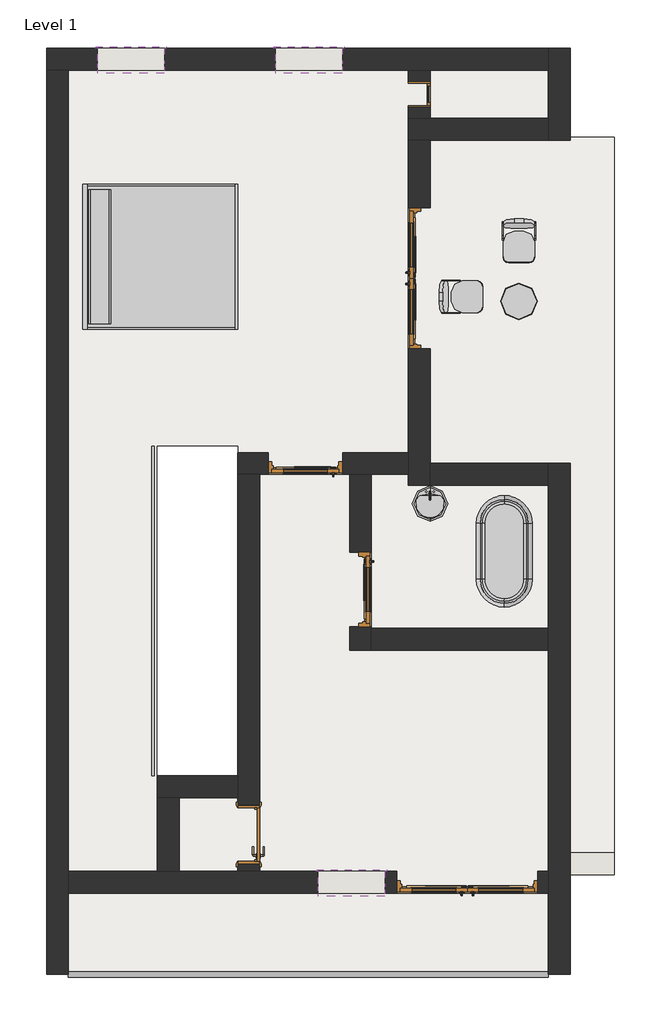
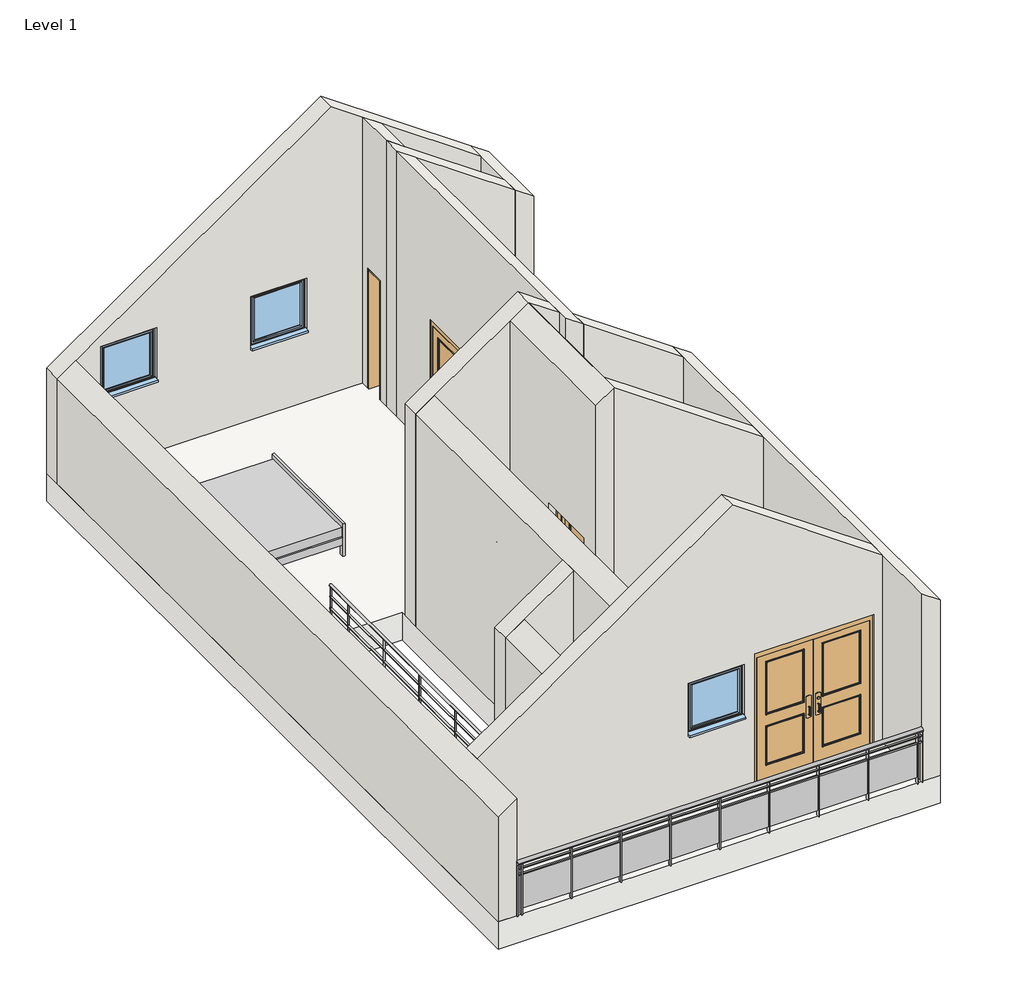
# One storey: 16 walls, 6 doors, 4 furniture elements, 3 windows, 2 flow terminals, 2 railings, 1 slab.
"""IFC4 building model written with IfcOpenShell, lengths in millimetres."""

from ifc_helpers import new_model, si_unit, point, frame, frame_2d, origin, place, context, project, spatial, polyline, circle_curve, ellipse_curve, trimmed, segment, composite_curve, outline, extrude, faceted_brep, transform, mapped, element, save
from ifc_brep_helpers import plane_surface, extruded_surface, advanced_brep
from components import door_9a5dd369, door_exterior_double_two_lite_door_exterior_double_two_lite_aa7d30b3, door_exterior_double_two_lite_door_exterior_double_two_lite_6b883914, door_exterior_double_two_lite_door_exterior_double_two_lite_037690dd, door_exterior_single_two_lite_door_exterior_single_two_lite_eb677f4d, doors_intsgl_810x2110mm_8206dd41, flow_terminal_a43f4bde, flow_terminal_0c5ffde2, furniture_b8e5f23d, furniture_eb3a3c23, furniture_9d41381f, windows_sgl_plain_910x910mm_cb8bb1e6

model = new_model("IFC4")

# Units and contexts
model_context = context("Model", 3, world=origin())
ifc_project = project(units=[si_unit("LENGTHUNIT", "METRE", prefix="MILLI")], contexts=[model_context])

# Site, building, storey
site = spatial("IfcSite", under=ifc_project)
building = spatial("IfcBuilding", under=site)
storey = spatial("IfcBuildingStorey", under=building, Name="Level 1", Elevation=3200.0)

# Doors
placement = place(None, origin())
door_shape = door_9a5dd369(model_context)
element("IfcDoor", 1, ObjectType="12\" x 80\"", at=placement, inside=storey, context=model_context, shape_type="MappedRepresentation", body=[
    mapped(door_shape, transform((-3132.0250057, 19503.7490528, 3200.0), x_axis=(0.0, -1.0, 0.0), y_axis=(1.0, 0.0, 0.0), z_axis=(0.0, 0.0, 1.0))),
])
door_exterior_double_two_lite_door_exterior_double_two_lite_shape = door_exterior_double_two_lite_door_exterior_double_two_lite_aa7d30b3(model_context)
door_exterior_double_two_lite_door_exterior_double_two_lite_2_shape = door_exterior_double_two_lite_door_exterior_double_two_lite_6b883914(model_context)
door_exterior_double_two_lite_door_exterior_double_two_lite_3_shape = door_exterior_double_two_lite_door_exterior_double_two_lite_037690dd(model_context)
element("IfcDoor", 2, ObjectType="Door-Exterior-Double-Two_Lite : Door-Exterior-Double-Two_Lite", at=placement, inside=storey, context=model_context, shape_type="MappedRepresentation", body=[
    mapped(door_exterior_double_two_lite_door_exterior_double_two_lite_shape, transform((-3128.8500057, 16990.7490528, 3200.0), x_axis=(0.0, 1.0, 0.0), y_axis=(-1.0, 0.0, 0.0), z_axis=(0.0, 0.0, 1.0))),
    mapped(door_exterior_double_two_lite_door_exterior_double_two_lite_2_shape, transform((-3128.8500057, 16990.7490528, 3200.0), x_axis=(0.0, 1.0, 0.0), y_axis=(-1.0, 0.0, 0.0), z_axis=(0.0, 0.0, 1.0))),
    mapped(door_exterior_double_two_lite_door_exterior_double_two_lite_3_shape, transform((-3128.8500057, 16990.7490528, 3200.0), x_axis=(0.0, 1.0, 0.0), y_axis=(-1.0, 0.0, 0.0), z_axis=(0.0, 0.0, 1.0))),
])
element("IfcDoor", 3, ObjectType="Door-Exterior-Double-Two_Lite : Door-Exterior-Double-Two_Lite", at=placement, inside=storey, context=model_context, shape_type="MappedRepresentation", body=[
    mapped(door_exterior_double_two_lite_door_exterior_double_two_lite_shape, transform((-2475.6750057, 8741.3490528, 3200.0), x_axis=(-1.0, 0.0, 0.0), y_axis=(0.0, -1.0, 0.0), z_axis=(0.0, 0.0, 1.0))),
    mapped(door_exterior_double_two_lite_door_exterior_double_two_lite_2_shape, transform((-2475.6750057, 8741.3490528, 3200.0), x_axis=(-1.0, 0.0, 0.0), y_axis=(0.0, -1.0, 0.0), z_axis=(0.0, 0.0, 1.0))),
    mapped(door_exterior_double_two_lite_door_exterior_double_two_lite_3_shape, transform((-2475.6750057, 8741.3490528, 3200.0), x_axis=(-1.0, 0.0, 0.0), y_axis=(0.0, -1.0, 0.0), z_axis=(0.0, 0.0, 1.0))),
])
door_exterior_single_two_lite_door_exterior_single_two_lite_shape = door_exterior_single_two_lite_door_exterior_single_two_lite_eb677f4d(model_context)
element("IfcDoor", 4, ObjectType="Door-Exterior-Single-Two_Lite : Door-Exterior-Single-Two_Lite", at=placement, inside=storey, context=model_context, shape_type="MappedRepresentation", body=[
    mapped(door_exterior_single_two_lite_door_exterior_single_two_lite_shape, transform((-4688.1750057, 14466.3490528, 3200.0), x_axis=(-1.0, 0.0, 0.0), y_axis=(0.0, -1.0, 0.0), z_axis=(0.0, 0.0, 1.0))),
])
element("IfcDoor", 5, ObjectType="Door-Exterior-Single-Two_Lite : Door-Exterior-Single-Two_Lite", at=placement, inside=storey, context=model_context, shape_type="MappedRepresentation", body=[
    mapped(door_exterior_single_two_lite_door_exterior_single_two_lite_shape, transform((-3941.5500057, 12737.0490528, 3200.0), x_axis=(0.0, -1.0, 0.0), y_axis=(1.0, 0.0, 0.0), z_axis=(0.0, 0.0, 1.0))),
])
doors_intsgl_810x2110mm_shape = doors_intsgl_810x2110mm_8206dd41(model_context)
element("IfcDoor", 6, ObjectType="Doors_IntSgl : 810x2110mm", at=placement, inside=storey, context=model_context, shape_type="MappedRepresentation", body=[
    mapped(doors_intsgl_810x2110mm_shape, transform((-5460.2000057, 9388.7490528, 3200.0), x_axis=(0.0, 1.0, 0.0), y_axis=(-1.0, 0.0, 0.0), z_axis=(0.0, 0.0, 1.0))),
])

# Flow terminals
flow_terminal_shape = flow_terminal_a43f4bde(model_context)
element("IfcFlowTerminal", 7, ObjectType="Sink Vanity-Round : 19\" x 19\"", at=placement, inside=storey, context=model_context, shape_type="MappedRepresentation", body=[
    mapped(flow_terminal_shape, transform((-3081.8517463, 13827.6587105, 3200.0), x_axis=(1.0, 0.0, 0.0), y_axis=(0.0, 1.0, 0.0), z_axis=(0.0, 0.0, 1.0))),
])
flow_terminal_2_shape = flow_terminal_0c5ffde2(model_context)
element("IfcFlowTerminal", 8, ObjectType="Tub-Free Standing-3D : 30\" x 60\"", at=placement, inside=storey, context=model_context, shape_type="MappedRepresentation", body=[
    mapped(flow_terminal_2_shape, transform((-1970.2000057, 13259.9990528, 3200.0), x_axis=(1.0, 0.0, 0.0), y_axis=(0.0, 1.0, 0.0), z_axis=(0.0, 0.0, 1.0))),
])

# Furniture
furniture_shape = furniture_b8e5f23d(model_context)
element("IfcFurniture", 9, ObjectType="Bed-Shaker : King 78\" x 83\"", at=placement, inside=storey, context=model_context, shape_type="MappedRepresentation", body=[
    mapped(furniture_shape, transform((-7718.4000057, 17303.4490528, 3200.0), x_axis=(0.0, 1.0, 0.0), y_axis=(-1.0, 0.0, 0.0), z_axis=(0.0, 0.0, 1.0))),
])
furniture_2_shape = furniture_eb3a3c23(model_context)
element("IfcFurniture", 10, ObjectType="Seating-Auditorium : 18\" x 24\" x 30\"", at=placement, inside=storey, context=model_context, shape_type="MappedRepresentation", body=[
    mapped(furniture_2_shape, transform((-2760.0754155, 16899.3269216, 3200.0), x_axis=(0.0, -1.0, 0.0), y_axis=(1.0, 0.0, 0.0), z_axis=(0.0, 0.0, 1.0))),
])
element("IfcFurniture", 11, ObjectType="Seating-Auditorium : 18\" x 24\" x 30\"", at=placement, inside=storey, context=model_context, shape_type="MappedRepresentation", body=[
    mapped(furniture_2_shape, transform((-1609.4721368, 17699.8744626, 3200.0), x_axis=(-1.0, 0.0, 0.0), y_axis=(0.0, -1.0, 0.0), z_axis=(0.0, 0.0, 1.0))),
])
furniture_3_shape = furniture_9d41381f(model_context)
element("IfcFurniture", 12, ObjectType="Table-Trio End : 20\" Diameter", at=placement, inside=storey, context=model_context, shape_type="MappedRepresentation", body=[
    mapped(furniture_3_shape, transform((-1770.2000057, 16674.9990528, 3200.0), x_axis=(1.0, 0.0, 0.0), y_axis=(0.0, 1.0, 0.0), z_axis=(0.0, 0.0, 1.0))),
])

# Railings
element("IfcRailing", 13, ObjectType="900mm_Pipe", at=placement, inside=storey, context=model_context, shape_type="SweptSolid", body=[
    extrude(outline(composite_curve([segment(trimmed(circle_curve(frame_2d((4080.0, -6770.2000057)), 20.0), [point((4080.0, -6750.2000057))], [point((4080.0, -6790.2000057))], False, "CARTESIAN"), True, "CONTINUOUS"), segment(trimmed(circle_curve(frame_2d((4080.0, -6770.2000057)), 20.0), [point((4080.0, -6790.2000057))], [point((4080.0, -6750.2000057))], False, "CARTESIAN"), True, "CONTINUOUS")], self_intersect=False)), frame((0.0, 10192.4990528, 0.0), z_axis=(0.0, 1.0, 0.0), x_axis=(0.0, 0.0, 1.0)), (0.0, 0.0, 1.0), 4500.0),
    extrude(outline(composite_curve([segment(trimmed(circle_curve(frame_2d((3885.0, -6770.2000057)), 15.0), [point((3885.0, -6785.2000057))], [point((3885.0, -6755.2000057))], False, "CARTESIAN"), True, "CONTINUOUS"), segment(trimmed(circle_curve(frame_2d((3885.0, -6770.2000057)), 15.0), [point((3885.0, -6755.2000057))], [point((3885.0, -6785.2000057))], False, "CARTESIAN"), True, "CONTINUOUS")], self_intersect=False)), frame((0.0, 10192.4990528, 0.0), z_axis=(0.0, 1.0, 0.0), x_axis=(0.0, 0.0, 1.0)), (0.0, 0.0, 1.0), 4500.0),
    extrude(outline(composite_curve([segment(trimmed(circle_curve(frame_2d((3685.0, -6770.2000057)), 15.0), [point((3685.0, -6785.2000057))], [point((3685.0, -6755.2000057))], False, "CARTESIAN"), True, "CONTINUOUS"), segment(trimmed(circle_curve(frame_2d((3685.0, -6770.2000057)), 15.0), [point((3685.0, -6755.2000057))], [point((3685.0, -6785.2000057))], False, "CARTESIAN"), True, "CONTINUOUS")], self_intersect=False)), frame((0.0, 10192.4990528, 0.0), z_axis=(0.0, 1.0, 0.0), x_axis=(0.0, 0.0, 1.0)), (0.0, 0.0, 1.0), 4500.0),
    extrude(outline(composite_curve([segment(trimmed(circle_curve(frame_2d((3485.0, -6770.2000057)), 15.0), [point((3485.0, -6785.2000057))], [point((3485.0, -6755.2000057))], False, "CARTESIAN"), True, "CONTINUOUS"), segment(trimmed(circle_curve(frame_2d((3485.0, -6770.2000057)), 15.0), [point((3485.0, -6755.2000057))], [point((3485.0, -6785.2000057))], False, "CARTESIAN"), True, "CONTINUOUS")], self_intersect=False)), frame((0.0, 10192.4990528, 0.0), z_axis=(0.0, 1.0, 0.0), x_axis=(0.0, 0.0, 1.0)), (0.0, 0.0, 1.0), 4500.0),
    extrude(outline(composite_curve([segment(trimmed(circle_curve(frame_2d((3285.0, -6770.2000057)), 15.0), [point((3285.0, -6785.2000057))], [point((3285.0, -6755.2000057))], False, "CARTESIAN"), True, "CONTINUOUS"), segment(trimmed(circle_curve(frame_2d((3285.0, -6770.2000057)), 15.0), [point((3285.0, -6755.2000057))], [point((3285.0, -6785.2000057))], False, "CARTESIAN"), True, "CONTINUOUS")], self_intersect=False)), frame((0.0, 10192.4990528, 0.0), z_axis=(0.0, 1.0, 0.0), x_axis=(0.0, 0.0, 1.0)), (0.0, 0.0, 1.0), 4500.0),
    extrude(outline(composite_curve([segment(trimmed(circle_curve(frame_2d((-6770.2000057, 14192.4990528)), 12.5), [point((-6782.7000057, 14192.4990528))], [point((-6757.7000057, 14192.4990528))], False, "CARTESIAN"), True, "CONTINUOUS"), segment(trimmed(circle_curve(frame_2d((-6770.2000057, 14192.4990528)), 12.5), [point((-6757.7000057, 14192.4990528))], [point((-6782.7000057, 14192.4990528))], False, "CARTESIAN"), True, "CONTINUOUS")], self_intersect=False)), frame((0.0, 0.0, 3200.0), z_axis=(0.0, 0.0, 1.0), x_axis=(1.0, 0.0, 0.0)), (0.0, 0.0, 1.0), 860.0),
    extrude(outline(composite_curve([segment(trimmed(circle_curve(frame_2d((-6770.2000057, 13192.4990528)), 12.5), [point((-6782.7000057, 13192.4990528))], [point((-6757.7000057, 13192.4990528))], False, "CARTESIAN"), True, "CONTINUOUS"), segment(trimmed(circle_curve(frame_2d((-6770.2000057, 13192.4990528)), 12.5), [point((-6757.7000057, 13192.4990528))], [point((-6782.7000057, 13192.4990528))], False, "CARTESIAN"), True, "CONTINUOUS")], self_intersect=False)), frame((0.0, 0.0, 3200.0), z_axis=(0.0, 0.0, 1.0), x_axis=(1.0, 0.0, 0.0)), (0.0, 0.0, 1.0), 860.0),
    extrude(outline(composite_curve([segment(trimmed(circle_curve(frame_2d((-6770.2000057, 12192.4990528)), 12.5), [point((-6782.7000057, 12192.4990528))], [point((-6757.7000057, 12192.4990528))], False, "CARTESIAN"), True, "CONTINUOUS"), segment(trimmed(circle_curve(frame_2d((-6770.2000057, 12192.4990528)), 12.5), [point((-6757.7000057, 12192.4990528))], [point((-6782.7000057, 12192.4990528))], False, "CARTESIAN"), True, "CONTINUOUS")], self_intersect=False)), frame((0.0, 0.0, 3200.0), z_axis=(0.0, 0.0, 1.0), x_axis=(1.0, 0.0, 0.0)), (0.0, 0.0, 1.0), 860.0),
    extrude(outline(composite_curve([segment(trimmed(circle_curve(frame_2d((-6770.2000057, 11192.4990528)), 12.5), [point((-6782.7000057, 11192.4990528))], [point((-6757.7000057, 11192.4990528))], False, "CARTESIAN"), True, "CONTINUOUS"), segment(trimmed(circle_curve(frame_2d((-6770.2000057, 11192.4990528)), 12.5), [point((-6757.7000057, 11192.4990528))], [point((-6782.7000057, 11192.4990528))], False, "CARTESIAN"), True, "CONTINUOUS")], self_intersect=False)), frame((0.0, 0.0, 3200.0), z_axis=(0.0, 0.0, 1.0), x_axis=(1.0, 0.0, 0.0)), (0.0, 0.0, 1.0), 860.0),
    extrude(outline(composite_curve([segment(trimmed(circle_curve(frame_2d((-6770.2000057, 14679.9990528)), 12.5), [point((-6782.7000057, 14679.9990528))], [point((-6757.7000057, 14679.9990528))], False, "CARTESIAN"), True, "CONTINUOUS"), segment(trimmed(circle_curve(frame_2d((-6770.2000057, 14679.9990528)), 12.5), [point((-6757.7000057, 14679.9990528))], [point((-6782.7000057, 14679.9990528))], False, "CARTESIAN"), True, "CONTINUOUS")], self_intersect=False)), frame((0.0, 0.0, 3200.0), z_axis=(0.0, 0.0, 1.0), x_axis=(1.0, 0.0, 0.0)), (0.0, 0.0, 1.0), 860.0),
    extrude(outline(composite_curve([segment(trimmed(circle_curve(frame_2d((-6770.2000057, 10204.9990528)), 12.5), [point((-6782.7000057, 10204.9990528))], [point((-6757.7000057, 10204.9990528))], False, "CARTESIAN"), True, "CONTINUOUS"), segment(trimmed(circle_curve(frame_2d((-6770.2000057, 10204.9990528)), 12.5), [point((-6757.7000057, 10204.9990528))], [point((-6782.7000057, 10204.9990528))], False, "CARTESIAN"), True, "CONTINUOUS")], self_intersect=False)), frame((0.0, 0.0, 3200.0), z_axis=(0.0, 0.0, 1.0), x_axis=(1.0, 0.0, 0.0)), (0.0, 0.0, 1.0), 860.0),
])
element("IfcRailing", 14, ObjectType="Glass_Panel-Bottom_Fill", at=placement, inside=storey, context=model_context, shape_type="SolidModel", body=[
    advanced_brep(
    [(-7925.2000057, 7516.889818, 4100.0), (-7925.2000057, 7436.889818, 4100.0), (-1370.2000057, 7516.889818, 4100.0), (-1370.2000057, 7436.889818, 4100.0)],
    [
        (0, 1, ellipse_curve(frame((-7925.2000057, 7476.889818, 4100.0), z_axis=(-1.0, 0.0, 0.0), x_axis=(0.0, -1.0, 0.0)), 40.0, 30.0)),
        (1, 0, ellipse_curve(frame((-7925.2000057, 7476.889818, 4100.0), z_axis=(-1.0, 0.0, 0.0), x_axis=(0.0, -1.0, 0.0)), 40.0, 30.0)),
        (2, 3, ellipse_curve(frame((-1370.2000057, 7476.889818, 4100.0), z_axis=(1.0, 0.0, 0.0), x_axis=(0.0, -1.0, 0.0)), 40.0, 30.0)),
        (3, 2, ellipse_curve(frame((-1370.2000057, 7476.889818, 4100.0), z_axis=(1.0, 0.0, 0.0), x_axis=(0.0, -1.0, 0.0)), 40.0, 30.0)),
        (0, 2),
        (3, 1),
    ],
    [
        plane_surface(frame((-7925.2000057, 7476.889818, 4100.0), z_axis=(-1.0, 0.0, 0.0), x_axis=(0.0, 1.0, 0.0))),
        plane_surface(frame((-1370.2000057, 7476.889818, 4100.0), z_axis=(1.0, 0.0, 0.0), x_axis=(0.0, 1.0, 0.0))),
        extruded_surface(trimmed(ellipse_curve(frame((-1370.2000057, 7476.889818, 4100.0), z_axis=(-1.0, 0.0, 0.0), x_axis=(0.0, -1.0, 0.0)), 40.0, 30.0), [point((-1370.2000057, 7516.889818, 4100.0))], [point((-1370.2000057, 7436.889818, 4100.0))], True, "CARTESIAN"), (-6555.0, 0.0, 0.0), 6555.0),
        extruded_surface(trimmed(ellipse_curve(frame((-1370.2000057, 7476.889818, 4100.0), z_axis=(-1.0, 0.0, 0.0), x_axis=(0.0, -1.0, 0.0)), 40.0, 30.0), [point((-1370.2000057, 7436.889818, 4100.0))], [point((-1370.2000057, 7516.889818, 4100.0))], True, "CARTESIAN"), (-6555.0, 0.0, 0.0), 6555.0),
    ],
    [
        (0, [[1, 2]]),
        (1, [[3, 4]]),
        (2, [[-1, 5, -4, 6]]),
        (3, [[-2, -6, -3, -5]]),
    ],
),
    extrude(outline(polyline([(-7925.2000057, 7467.4990528), (-7925.2000057, 7487.4990528), (-1370.2000057, 7487.4990528), (-1370.2000057, 7467.4990528), (-7925.2000057, 7467.4990528)])), frame((0.0, 0.0, 3980.0), z_axis=(0.0, 0.0, 1.0), x_axis=(1.0, 0.0, 0.0)), (0.0, 0.0, 1.0), 20.0),
    extrude(outline(polyline([(-7925.2000057, 7467.4990528), (-7925.2000057, 7487.4990528), (-1370.2000057, 7487.4990528), (-1370.2000057, 7467.4990528), (-7925.2000057, 7467.4990528)])), frame((0.0, 0.0, 3880.0), z_axis=(0.0, 0.0, 1.0), x_axis=(1.0, 0.0, 0.0)), (0.0, 0.0, 1.0), 20.0),
    extrude(outline(polyline([(-1453.7000057, 7502.4990528), (-1441.7000057, 7502.4990528), (-1441.7000057, 7452.4990528), (-1453.7000057, 7452.4990528), (-1453.7000057, 7502.4990528)])), frame((0.0, 0.0, 3200.0), z_axis=(0.0, 0.0, 1.0), x_axis=(1.0, 0.0, 0.0)), (0.0, 0.0, 1.0), 870.0),
    extrude(outline(polyline([(-2247.7000057, 7475.7742427), (-1447.7000057, 7475.7742427), (-1447.7000057, 7470.7742427), (-2247.7000057, 7470.7742427), (-2247.7000057, 7475.7742427)])), frame((0.0, 0.0, 3300.0), z_axis=(0.0, 0.0, 1.0), x_axis=(1.0, 0.0, 0.0)), (0.0, 0.0, 1.0), 580.0),
    extrude(outline(polyline([(-2253.7000057, 7502.4990528), (-2241.7000057, 7502.4990528), (-2241.7000057, 7452.4990528), (-2253.7000057, 7452.4990528), (-2253.7000057, 7502.4990528)])), frame((0.0, 0.0, 3200.0), z_axis=(0.0, 0.0, 1.0), x_axis=(1.0, 0.0, 0.0)), (0.0, 0.0, 1.0), 870.0),
    extrude(outline(polyline([(-3047.7000057, 7475.7742427), (-2247.7000057, 7475.7742427), (-2247.7000057, 7470.7742427), (-3047.7000057, 7470.7742427), (-3047.7000057, 7475.7742427)])), frame((0.0, 0.0, 3300.0), z_axis=(0.0, 0.0, 1.0), x_axis=(1.0, 0.0, 0.0)), (0.0, 0.0, 1.0), 580.0),
    extrude(outline(polyline([(-3053.7000057, 7502.4990528), (-3041.7000057, 7502.4990528), (-3041.7000057, 7452.4990528), (-3053.7000057, 7452.4990528), (-3053.7000057, 7502.4990528)])), frame((0.0, 0.0, 3200.0), z_axis=(0.0, 0.0, 1.0), x_axis=(1.0, 0.0, 0.0)), (0.0, 0.0, 1.0), 870.0),
    extrude(outline(polyline([(-3847.7000057, 7475.7742427), (-3047.7000057, 7475.7742427), (-3047.7000057, 7470.7742427), (-3847.7000057, 7470.7742427), (-3847.7000057, 7475.7742427)])), frame((0.0, 0.0, 3300.0), z_axis=(0.0, 0.0, 1.0), x_axis=(1.0, 0.0, 0.0)), (0.0, 0.0, 1.0), 580.0),
    extrude(outline(polyline([(-3853.7000057, 7502.4990528), (-3841.7000057, 7502.4990528), (-3841.7000057, 7452.4990528), (-3853.7000057, 7452.4990528), (-3853.7000057, 7502.4990528)])), frame((0.0, 0.0, 3200.0), z_axis=(0.0, 0.0, 1.0), x_axis=(1.0, 0.0, 0.0)), (0.0, 0.0, 1.0), 870.0),
    extrude(outline(polyline([(-4647.7000057, 7475.7742427), (-3847.7000057, 7475.7742427), (-3847.7000057, 7470.7742427), (-4647.7000057, 7470.7742427), (-4647.7000057, 7475.7742427)])), frame((0.0, 0.0, 3300.0), z_axis=(0.0, 0.0, 1.0), x_axis=(1.0, 0.0, 0.0)), (0.0, 0.0, 1.0), 580.0),
    extrude(outline(polyline([(-4653.7000057, 7502.4990528), (-4641.7000057, 7502.4990528), (-4641.7000057, 7452.4990528), (-4653.7000057, 7452.4990528), (-4653.7000057, 7502.4990528)])), frame((0.0, 0.0, 3200.0), z_axis=(0.0, 0.0, 1.0), x_axis=(1.0, 0.0, 0.0)), (0.0, 0.0, 1.0), 870.0),
    extrude(outline(polyline([(-5447.7000057, 7475.7742427), (-4647.7000057, 7475.7742427), (-4647.7000057, 7470.7742427), (-5447.7000057, 7470.7742427), (-5447.7000057, 7475.7742427)])), frame((0.0, 0.0, 3300.0), z_axis=(0.0, 0.0, 1.0), x_axis=(1.0, 0.0, 0.0)), (0.0, 0.0, 1.0), 580.0),
    extrude(outline(polyline([(-5453.7000057, 7502.4990528), (-5441.7000057, 7502.4990528), (-5441.7000057, 7452.4990528), (-5453.7000057, 7452.4990528), (-5453.7000057, 7502.4990528)])), frame((0.0, 0.0, 3200.0), z_axis=(0.0, 0.0, 1.0), x_axis=(1.0, 0.0, 0.0)), (0.0, 0.0, 1.0), 870.0),
    extrude(outline(polyline([(-6247.7000057, 7475.7742427), (-5447.7000057, 7475.7742427), (-5447.7000057, 7470.7742427), (-6247.7000057, 7470.7742427), (-6247.7000057, 7475.7742427)])), frame((0.0, 0.0, 3300.0), z_axis=(0.0, 0.0, 1.0), x_axis=(1.0, 0.0, 0.0)), (0.0, 0.0, 1.0), 580.0),
    extrude(outline(polyline([(-6253.7000057, 7502.4990528), (-6241.7000057, 7502.4990528), (-6241.7000057, 7452.4990528), (-6253.7000057, 7452.4990528), (-6253.7000057, 7502.4990528)])), frame((0.0, 0.0, 3200.0), z_axis=(0.0, 0.0, 1.0), x_axis=(1.0, 0.0, 0.0)), (0.0, 0.0, 1.0), 870.0),
    extrude(outline(polyline([(-7047.7000057, 7475.7742427), (-6247.7000057, 7475.7742427), (-6247.7000057, 7470.7742427), (-7047.7000057, 7470.7742427), (-7047.7000057, 7475.7742427)])), frame((0.0, 0.0, 3300.0), z_axis=(0.0, 0.0, 1.0), x_axis=(1.0, 0.0, 0.0)), (0.0, 0.0, 1.0), 580.0),
    extrude(outline(polyline([(-7053.7000057, 7502.4990528), (-7041.7000057, 7502.4990528), (-7041.7000057, 7452.4990528), (-7053.7000057, 7452.4990528), (-7053.7000057, 7502.4990528)])), frame((0.0, 0.0, 3200.0), z_axis=(0.0, 0.0, 1.0), x_axis=(1.0, 0.0, 0.0)), (0.0, 0.0, 1.0), 870.0),
    extrude(outline(polyline([(-7847.7000057, 7475.7742427), (-7047.7000057, 7475.7742427), (-7047.7000057, 7470.7742427), (-7847.7000057, 7470.7742427), (-7847.7000057, 7475.7742427)])), frame((0.0, 0.0, 3300.0), z_axis=(0.0, 0.0, 1.0), x_axis=(1.0, 0.0, 0.0)), (0.0, 0.0, 1.0), 580.0),
    extrude(outline(polyline([(-7853.7000057, 7502.4990528), (-7841.7000057, 7502.4990528), (-7841.7000057, 7452.4990528), (-7853.7000057, 7452.4990528), (-7853.7000057, 7502.4990528)])), frame((0.0, 0.0, 3200.0), z_axis=(0.0, 0.0, 1.0), x_axis=(1.0, 0.0, 0.0)), (0.0, 0.0, 1.0), 870.0),
    extrude(outline(polyline([(-1378.2000057, 7502.4990528), (-1366.2000057, 7502.4990528), (-1366.2000057, 7452.4990528), (-1378.2000057, 7452.4990528), (-1378.2000057, 7502.4990528)])), frame((0.0, 0.0, 3200.0), z_axis=(0.0, 0.0, 1.0), x_axis=(1.0, 0.0, 0.0)), (0.0, 0.0, 1.0), 870.0),
    extrude(outline(polyline([(-7929.2000057, 7502.4990528), (-7917.2000057, 7502.4990528), (-7917.2000057, 7452.4990528), (-7929.2000057, 7452.4990528), (-7929.2000057, 7502.4990528)])), frame((0.0, 0.0, 3200.0), z_axis=(0.0, 0.0, 1.0), x_axis=(1.0, 0.0, 0.0)), (0.0, 0.0, 1.0), 870.0),
])

# Slab
element("IfcSlab", 15, ObjectType="floor generic 150mm", at=placement, inside=storey, context=model_context, shape_type="SweptSolid", body=[
    extrude(outline(polyline([(-8225.2000057, 20132.4990528), (-1070.2000057, 20132.4990528), (-1070.2000057, 18917.4990528), (-470.2000057, 18917.4990528), (-470.2000057, 8842.4990528), (-481.4492748, 8842.4990528), (-1070.2000057, 8842.4990528), (-1070.2000057, 7477.4990528), (-8225.2000057, 7477.4990528), (-8225.2000057, 20132.4990528)]), holes=[polyline([(-5610.2000057, 14692.4990528), (-6710.2000057, 14692.4990528), (-6710.2000057, 10192.4990528), (-5610.2000057, 10192.4990528), (-5610.2000057, 14692.4990528)])]), frame((0.0, 0.0, 2730.0), z_axis=(0.0, 0.0, 1.0), x_axis=(1.0, 0.0, 0.0)), (0.0, 0.0, 1.0), 470.0),
])

# Walls
element("IfcWall", 16, at=placement, inside=storey, context=model_context, shape_type="Brep", body=[
    faceted_brep([(-2985.2000057, 19832.4990528, 3200.0), (-2985.2000057, 19832.4990528, 7540.8974357), (-2985.2000057, 19174.9990528, 7540.8974357), (-2985.2000057, 19174.9990528, 3200.0), (-2985.2000057, 19325.9490528, 3200.0), (-2985.2000057, 19325.9490528, 5257.4), (-2985.2000057, 19681.5490528, 5257.4), (-2985.2000057, 19681.5490528, 3200.0), (-3285.2000057, 19832.4990528, 7750.9596971), (-3285.2000057, 19832.4990528, 3200.0), (-3285.2000057, 19681.5490528, 3200.0), (-3285.2000057, 19681.5490528, 5257.4), (-3285.2000057, 19325.9490528, 5257.4), (-3285.2000057, 19325.9490528, 3200.0), (-3285.2000057, 19174.9990528, 3200.0), (-3285.2000057, 19174.9990528, 7750.9596971)], [[[0, 1, 2, 3, 4, 5, 6, 7]], [[8, 9, 10, 11, 12, 13, 14, 15]], [[3, 14, 13, 4]], [[9, 0, 7, 10]], [[1, 0, 9, 8]], [[3, 2, 15, 14]], [[12, 5, 4, 13]], [[6, 11, 10, 7]], [[2, 1, 8, 15]], [[11, 6, 5, 12]]]),
])
element("IfcWall", 17, at=placement, inside=storey, context=model_context, shape_type="Brep", body=[
    faceted_brep([(-3285.2000057, 14609.9990528, 7750.9596971), (-3285.2000057, 14609.9990528, 3200.0), (-4180.1750057, 14609.9990528, 3200.0), (-4180.1750057, 14609.9990528, 5435.2), (-5196.1750057, 14609.9990528, 5435.2), (-5196.1750057, 14609.9990528, 3200.0), (-5610.2000057, 14609.9990528, 3200.0), (-5610.2000057, 14609.9990528, 6831.0427124), (-3790.8112016, 14609.9990528, 8104.9924679), (-3285.2000057, 14309.9990528, 3200.0), (-3285.2000057, 14309.9990528, 7750.9596971), (-3785.2000057, 14309.9990528, 8101.0634662), (-3790.8112016, 14309.9990528, 8104.9924679), (-4085.2000057, 14309.9990528, 7898.8592082), (-5310.2000057, 14309.9990528, 7041.1049739), (-5610.2000057, 14309.9990528, 6831.0427124), (-5610.2000057, 14309.9990528, 3200.0), (-5310.2000057, 14309.9990528, 3200.0), (-5196.1750057, 14309.9990528, 3200.0), (-5196.1750057, 14309.9990528, 5435.2), (-4180.1750057, 14309.9990528, 5435.2), (-4180.1750057, 14309.9990528, 3200.0), (-4085.2000057, 14309.9990528, 3200.0), (-3785.2000057, 14309.9990528, 3200.0)], [[[0, 1, 2, 3, 4, 5, 6, 7, 8]], [[9, 10, 11, 12, 13, 14, 15, 16, 17, 18, 19, 20, 21, 22, 23]], [[1, 9, 23, 22, 21, 2]], [[16, 6, 5, 18, 17]], [[1, 0, 10, 9]], [[7, 6, 16, 15]], [[4, 19, 18, 5]], [[20, 3, 2, 21]], [[10, 0, 8, 12, 11]], [[7, 15, 14, 13, 12, 8]], [[3, 20, 19, 4]]]),
])
element("IfcWall", 18, at=placement, inside=storey, context=model_context, shape_type="Brep", body=[
    faceted_brep([(-5610.2000057, 14309.9990528, 6831.0427124), (-5610.2000057, 14309.9990528, 3200.0), (-5610.2000057, 10192.4990528, 3200.0), (-5610.2000057, 9892.4990528, 3200.0), (-5610.2000057, 9793.7490528, 3200.0), (-5610.2000057, 9793.7490528, 5310.0), (-5610.2000057, 8983.7490528, 5310.0), (-5610.2000057, 8983.7490528, 3200.0), (-5610.2000057, 8884.9990528, 3200.0), (-5610.2000057, 8884.9990528, 6831.0427124), (-5610.2000057, 9892.4990528, 6831.0427124), (-5610.2000057, 10192.4990528, 6831.0427124), (-5310.2000057, 14309.9990528, 3200.0), (-5310.2000057, 14309.9990528, 7041.1049739), (-5310.2000057, 8884.9990528, 7041.1049739), (-5310.2000057, 8884.9990528, 3200.0), (-5310.2000057, 8983.7490528, 3200.0), (-5310.2000057, 8983.7490528, 5310.0), (-5310.2000057, 9793.7490528, 5310.0), (-5310.2000057, 9793.7490528, 3200.0)], [[[0, 1, 2, 3, 4, 5, 6, 7, 8, 9, 10, 11]], [[12, 13, 14, 15, 16, 17, 18, 19]], [[1, 12, 19, 4, 3, 2]], [[15, 8, 7, 16]], [[1, 0, 13, 12]], [[9, 8, 15, 14]], [[18, 5, 4, 19]], [[6, 17, 16, 7]], [[0, 11, 10, 9, 14, 13]], [[17, 6, 5, 18]]]),
])
element("IfcWall", 19, at=placement, inside=storey, context=model_context, shape_type="Brep", body=[
    faceted_brep([(-5610.2000057, 10192.4990528, 3200.0), (-6710.2000057, 10192.4990528, 3200.0), (-6710.2000057, 10192.4990528, 6060.8144204), (-5610.2000057, 10192.4990528, 6831.0427124), (-5610.2000057, 9892.4990528, 3200.0), (-5610.2000057, 9892.4990528, 6831.0427124), (-6410.2000057, 9892.4990528, 6270.8766819), (-6710.2000057, 9892.4990528, 6060.8144204), (-6710.2000057, 9892.4990528, 3200.0), (-6410.2000057, 9892.4990528, 3200.0)], [[[0, 1, 2, 3]], [[4, 5, 6, 7, 8, 9]], [[1, 0, 4, 9, 8]], [[0, 3, 5, 4]], [[2, 1, 8, 7]], [[3, 2, 7, 6, 5]]]),
])
element("IfcWall", 20, at=placement, inside=storey, context=model_context, shape_type="SweptSolid", body=[
    extrude(outline(polyline([(6060.8144204, -6710.2000057), (3200.0, -6710.2000057), (3200.0, -6410.2000057), (6270.8766819, -6410.2000057), (6060.8144204, -6710.2000057)])), frame((0.0, 8884.9990528, 0.0), z_axis=(0.0, 1.0, 0.0), x_axis=(0.0, 0.0, 1.0)), (0.0, 0.0, 1.0), 1007.5),
])
element("IfcWall", 21, at=placement, inside=storey, context=model_context, shape_type="Brep", body=[
    faceted_brep([(-4085.2000057, 14309.9990528, 7898.8592082), (-4085.2000057, 14309.9990528, 3200.0), (-4085.2000057, 13245.0490528, 3200.0), (-4085.2000057, 13245.0490528, 5435.2), (-4085.2000057, 12229.0490528, 5435.2), (-4085.2000057, 12229.0490528, 3200.0), (-4085.2000057, 11909.9990528, 3200.0), (-4085.2000057, 11909.9990528, 7898.8592082), (-3785.2000057, 14309.9990528, 8101.0634662), (-3785.2000057, 12209.9990528, 8101.0634662), (-3785.2000057, 11909.9990528, 8101.0634662), (-3785.2000057, 11909.9990528, 3200.0), (-3785.2000057, 12209.9990528, 3200.0), (-3785.2000057, 12229.0490528, 3200.0), (-3785.2000057, 12229.0490528, 5435.2), (-3785.2000057, 13245.0490528, 5435.2), (-3785.2000057, 13245.0490528, 3200.0), (-3785.2000057, 14309.9990528, 3200.0), (-3790.8112016, 14309.9990528, 8104.9924679), (-3790.8112016, 11909.9990528, 8104.9924679)], [[[0, 1, 2, 3, 4, 5, 6, 7]], [[8, 9, 10, 11, 12, 13, 14, 15, 16, 17]], [[1, 17, 16, 2]], [[11, 6, 5, 13, 12]], [[1, 0, 18, 8, 17]], [[7, 6, 11, 10, 19]], [[4, 14, 13, 5]], [[15, 3, 2, 16]], [[0, 7, 19, 18]], [[10, 9, 8, 18, 19]], [[3, 15, 14, 4]]]),
])
element("IfcWall", 22, at=placement, inside=storey, context=model_context, shape_type="SweptSolid", body=[
    extrude(outline(polyline([(3200.0, -3785.2000057), (3200.0, -1370.2000057), (6410.0622615, -1370.2000057), (8101.0634662, -3785.2000057), (3200.0, -3785.2000057)])), frame((0.0, 11909.9990528, 0.0), z_axis=(0.0, 1.0, 0.0), x_axis=(0.0, 0.0, 1.0)), (0.0, 0.0, 1.0), 300.0),
])
element("IfcWall", 23, at=placement, inside=storey, context=model_context, shape_type="Brep", body=[
    faceted_brep([(-1070.2000057, 8842.4990528, 3200.0), (-470.2000057, 8842.4990528, 3200.0), (-470.2000057, 8842.4990528, 4100.0), (-470.2000057, 8842.4990528, 4104.0395842), (-1070.2000057, 8842.4990528, 4104.0395842), (-1070.2000057, 9142.4990528, 3200.0), (-1070.2000057, 9142.4990528, 4104.0395842), (-470.2000057, 9142.4990528, 4104.0395842), (-470.2000057, 9142.4990528, 3200.0)], [[[0, 1, 2, 3, 4]], [[5, 6, 7, 8]], [[1, 0, 5, 8]], [[4, 3, 7, 6]], [[3, 2, 1, 8, 7]], [[0, 4, 6, 5]]]),
])
element("IfcWall", 24, ObjectType="Wall-Ret_300Con", at=placement, inside=storey, context=model_context, shape_type="Brep", body=[
    faceted_brep([(-8225.2000057, 19832.4990528, 3200.0), (-7925.2000057, 19832.4990528, 3200.0), (-3285.2000057, 19832.4990528, 3200.0), (-2985.2000057, 19832.4990528, 3200.0), (-1370.2000057, 19832.4990528, 3200.0), (-1370.2000057, 19832.4990528, 6410.0622615), (-2985.2000057, 19832.4990528, 7540.8974357), (-3285.2000057, 19832.4990528, 7750.9596971), (-3790.8112016, 19832.4990528, 8104.9924679), (-7925.2000057, 19832.4990528, 5210.0622615), (-8225.2000057, 19832.4990528, 5000.0), (-6615.2000057, 19832.4990528, 5310.0), (-6615.2000057, 19832.4990528, 4400.0), (-7525.2000057, 19832.4990528, 4400.0), (-7525.2000057, 19832.4990528, 5310.0), (-4185.2000057, 19832.4990528, 5310.0), (-4185.2000057, 19832.4990528, 4400.0), (-5095.2000057, 19832.4990528, 4400.0), (-5095.2000057, 19832.4990528, 5310.0), (-1370.2000057, 20132.4990528, 3200.0), (-8225.2000057, 20132.4990528, 3200.0), (-8225.2000057, 20132.4990528, 5000.0), (-3790.8112016, 20132.4990528, 8104.9924679), (-1370.2000057, 20132.4990528, 6410.0622615), (-6615.2000057, 20132.4990528, 4400.0), (-6615.2000057, 20132.4990528, 5310.0), (-7525.2000057, 20132.4990528, 5310.0), (-7525.2000057, 20132.4990528, 4400.0), (-4185.2000057, 20132.4990528, 4400.0), (-4185.2000057, 20132.4990528, 5310.0), (-5095.2000057, 20132.4990528, 5310.0), (-5095.2000057, 20132.4990528, 4400.0)], [[[0, 1, 2, 3, 4, 5, 6, 7, 8, 9, 10], [11, 12, 13, 14], [15, 16, 17, 18]], [[19, 20, 21, 22, 23], [24, 25, 26, 27], [28, 29, 30, 31]], [[4, 3, 2, 1, 0, 20, 19]], [[0, 10, 21, 20]], [[5, 4, 19, 23]], [[24, 12, 11, 25]], [[12, 24, 27, 13]], [[13, 27, 26, 14]], [[15, 29, 28, 16]], [[16, 28, 31, 17]], [[17, 31, 30, 18]], [[21, 10, 9, 8, 22]], [[5, 23, 22, 8, 7, 6]], [[25, 11, 14, 26]], [[29, 15, 18, 30]]]),
])
element("IfcWall", 25, ObjectType="Wall-Ret_300Con", at=placement, inside=storey, context=model_context, shape_type="Brep", body=[
    faceted_brep([(-7925.2000057, 7477.4990528, 3200.0), (-7925.2000057, 8584.9990528, 3200.0), (-7925.2000057, 8884.9990528, 3200.0), (-7925.2000057, 19832.4990528, 3200.0), (-7925.2000057, 19832.4990528, 5210.0622615), (-7925.2000057, 8884.9990528, 5210.0622615), (-7925.2000057, 8584.9990528, 5210.0622615), (-7925.2000057, 7477.4990528, 5210.0622615), (-8225.2000057, 7477.4990528, 3200.0), (-8225.2000057, 7477.4990528, 5000.0), (-8225.2000057, 19832.4990528, 5000.0), (-8225.2000057, 19832.4990528, 3200.0)], [[[0, 1, 2, 3, 4, 5, 6, 7]], [[8, 9, 10, 11]], [[3, 2, 1, 0, 8, 11]], [[0, 7, 9, 8]], [[4, 3, 11, 10]], [[7, 6, 5, 4, 10, 9]]]),
])
element("IfcWall", 26, ObjectType="Wall-Ret_300Con", at=placement, inside=storey, context=model_context, shape_type="Brep", body=[
    faceted_brep([(-1370.2000057, 20132.4990528, 3200.0), (-1370.2000057, 19832.4990528, 3200.0), (-1370.2000057, 19174.9990528, 3200.0), (-1370.2000057, 18874.9990528, 3200.0), (-1370.2000057, 18874.9990528, 6410.0622615), (-1370.2000057, 19174.9990528, 6410.0622615), (-1370.2000057, 19832.4990528, 6410.0622615), (-1370.2000057, 20132.4990528, 6410.0622615), (-1070.2000057, 20132.4990528, 3200.0), (-1070.2000057, 20132.4990528, 6200.0), (-1070.2000057, 18874.9990528, 6200.0), (-1070.2000057, 18874.9990528, 3200.0)], [[[0, 1, 2, 3, 4, 5, 6, 7]], [[8, 9, 10, 11]], [[3, 2, 1, 0, 8, 11]], [[0, 7, 9, 8]], [[4, 3, 11, 10]], [[7, 6, 5, 4, 10, 9]]]),
])
element("IfcWall", 27, ObjectType="Wall-Ret_300Con", at=placement, inside=storey, context=model_context, shape_type="Brep", body=[
    faceted_brep([(-1370.2000057, 19174.9990528, 3200.0), (-2985.2000057, 19174.9990528, 3200.0), (-3285.2000057, 19174.9990528, 3200.0), (-3285.2000057, 19174.9990528, 7750.9596971), (-2985.2000057, 19174.9990528, 7540.8974357), (-1370.2000057, 19174.9990528, 6410.0622615), (-1370.2000057, 18874.9990528, 3200.0), (-1370.2000057, 18874.9990528, 6410.0622615), (-2985.2000057, 18874.9990528, 7540.8974357), (-3285.2000057, 18874.9990528, 7750.9596971), (-3285.2000057, 18874.9990528, 3200.0), (-2985.2000057, 18874.9990528, 3200.0)], [[[0, 1, 2, 3, 4, 5]], [[6, 7, 8, 9, 10, 11]], [[2, 1, 0, 6, 11, 10]], [[0, 5, 7, 6]], [[3, 2, 10, 9]], [[5, 4, 3, 9, 8, 7]]]),
])
element("IfcWall", 28, ObjectType="Wall-Ret_300Con", at=placement, inside=storey, context=model_context, shape_type="Brep", body=[
    faceted_brep([(-3285.2000057, 18874.9990528, 7750.9596971), (-3285.2000057, 18874.9990528, 3200.0), (-3285.2000057, 17955.9490528, 3200.0), (-3285.2000057, 17955.9490528, 5435.2), (-3285.2000057, 16025.5490528, 5435.2), (-3285.2000057, 16025.5490528, 3200.0), (-3285.2000057, 14609.9990528, 3200.0), (-3285.2000057, 14309.9990528, 3200.0), (-3285.2000057, 14159.9990528, 3200.0), (-3285.2000057, 14159.9990528, 7750.9596971), (-3285.2000057, 14309.9990528, 7750.9596971), (-3285.2000057, 14609.9990528, 7750.9596971), (-2985.2000057, 18874.9990528, 3200.0), (-2985.2000057, 18874.9990528, 7540.8974357), (-2985.2000057, 14459.9990528, 7540.8974357), (-2985.2000057, 14159.9990528, 7540.8974357), (-2985.2000057, 14159.9990528, 3200.0), (-2985.2000057, 14459.9990528, 3200.0), (-2985.2000057, 16025.5490528, 3200.0), (-2985.2000057, 16025.5490528, 5435.2), (-2985.2000057, 17955.9490528, 5435.2), (-2985.2000057, 17955.9490528, 3200.0)], [[[0, 1, 2, 3, 4, 5, 6, 7, 8, 9, 10, 11]], [[12, 13, 14, 15, 16, 17, 18, 19, 20, 21]], [[1, 12, 21, 2]], [[16, 8, 7, 6, 5, 18, 17]], [[1, 0, 13, 12]], [[9, 8, 16, 15]], [[20, 3, 2, 21]], [[4, 19, 18, 5]], [[13, 0, 11, 10, 9, 15, 14]], [[19, 4, 3, 20]]]),
])
element("IfcWall", 29, ObjectType="Wall-Ret_300Con", at=placement, inside=storey, context=model_context, shape_type="SweptSolid", body=[
    extrude(outline(polyline([(3200.0, -2985.2000057), (3200.0, -1370.2000057), (6410.0622615, -1370.2000057), (7540.8974357, -2985.2000057), (3200.0, -2985.2000057)])), frame((0.0, 14159.9990528, 0.0), z_axis=(0.0, 1.0, 0.0), x_axis=(0.0, 0.0, 1.0)), (0.0, 0.0, 1.0), 300.0),
])
element("IfcWall", 30, ObjectType="Wall-Ret_300Con", at=placement, inside=storey, context=model_context, shape_type="Brep", body=[
    faceted_brep([(-1370.2000057, 14459.9990528, 3200.0), (-1370.2000057, 14159.9990528, 3200.0), (-1370.2000057, 12209.9990528, 3200.0), (-1370.2000057, 11909.9990528, 3200.0), (-1370.2000057, 8884.9990528, 3200.0), (-1370.2000057, 8584.9990528, 3200.0), (-1370.2000057, 7477.4990528, 3200.0), (-1370.2000057, 7477.4990528, 6410.0622615), (-1370.2000057, 8584.9990528, 6410.0622615), (-1370.2000057, 8884.9990528, 6410.0622615), (-1370.2000057, 11909.9990528, 6410.0622615), (-1370.2000057, 12209.9990528, 6410.0622615), (-1370.2000057, 14159.9990528, 6410.0622615), (-1370.2000057, 14459.9990528, 6410.0622615), (-1070.2000057, 14459.9990528, 3200.0), (-1070.2000057, 14459.9990528, 6200.0), (-1070.2000057, 7477.4990528, 6200.0), (-1070.2000057, 7477.4990528, 3200.0), (-1070.2000057, 8842.4990528, 3200.0), (-1070.2000057, 9142.4990528, 3200.0)], [[[0, 1, 2, 3, 4, 5, 6, 7, 8, 9, 10, 11, 12, 13]], [[14, 15, 16, 17, 18, 19]], [[6, 5, 4, 3, 2, 1, 0, 14, 19, 18, 17]], [[7, 6, 17, 16]], [[0, 13, 15, 14]], [[13, 12, 11, 10, 9, 8, 7, 16, 15]]]),
])
element("IfcWall", 31, ObjectType="Wall-Ret_300Con", at=placement, inside=storey, context=model_context, shape_type="Brep", body=[
    faceted_brep([(-7925.2000057, 8884.9990528, 3200.0), (-7925.2000057, 8884.9990528, 5210.0622615), (-6710.2000057, 8884.9990528, 6060.8144204), (-6410.2000057, 8884.9990528, 6270.8766819), (-5610.2000057, 8884.9990528, 6831.0427124), (-5310.2000057, 8884.9990528, 7041.1049739), (-3790.8112016, 8884.9990528, 8104.9924679), (-1370.2000057, 8884.9990528, 6410.0622615), (-1370.2000057, 8884.9990528, 3200.0), (-1510.4750057, 8884.9990528, 3200.0), (-1510.4750057, 8884.9990528, 5435.2), (-3440.8750057, 8884.9990528, 5435.2), (-3440.8750057, 8884.9990528, 3200.0), (-5310.2000057, 8884.9990528, 3200.0), (-5610.2000057, 8884.9990528, 3200.0), (-6410.2000057, 8884.9990528, 3200.0), (-6710.2000057, 8884.9990528, 3200.0), (-3600.2000057, 8884.9990528, 4400.0), (-3600.2000057, 8884.9990528, 5310.0), (-4510.2000057, 8884.9990528, 5310.0), (-4510.2000057, 8884.9990528, 4400.0), (-7925.2000057, 8584.9990528, 5210.0622615), (-7925.2000057, 8584.9990528, 3200.0), (-3440.8750057, 8584.9990528, 3200.0), (-3440.8750057, 8584.9990528, 5435.2), (-1510.4750057, 8584.9990528, 5435.2), (-1510.4750057, 8584.9990528, 3200.0), (-1370.2000057, 8584.9990528, 3200.0), (-1370.2000057, 8584.9990528, 6410.0622615), (-3790.8112016, 8584.9990528, 8104.9924679), (-3600.2000057, 8584.9990528, 5310.0), (-3600.2000057, 8584.9990528, 4400.0), (-4510.2000057, 8584.9990528, 4400.0), (-4510.2000057, 8584.9990528, 5310.0)], [[[0, 1, 2, 3, 4, 5, 6, 7, 8, 9, 10, 11, 12, 13, 14, 15, 16], [17, 18, 19, 20]], [[21, 22, 23, 24, 25, 26, 27, 28, 29], [30, 31, 32, 33]], [[8, 27, 26, 9]], [[22, 0, 16, 15, 14, 13, 12, 23]], [[1, 0, 22, 21]], [[8, 7, 28, 27]], [[28, 7, 6, 29]], [[1, 21, 29, 6, 5, 4, 3, 2]], [[31, 30, 18, 17]], [[32, 31, 17, 20]], [[33, 32, 20, 19]], [[30, 33, 19, 18]], [[11, 24, 23, 12]], [[24, 11, 10, 25]], [[25, 10, 9, 26]]]),
])

# Windows
windows_sgl_plain_910x910mm_shape = windows_sgl_plain_910x910mm_cb8bb1e6(model_context)
element("IfcWindow", 32, ObjectType="Windows_Sgl_Plain : 910x910mm", at=placement, inside=storey, context=model_context, shape_type="MappedRepresentation", body=[
    mapped(windows_sgl_plain_910x910mm_shape, transform((-7070.2000057, 19990.9556206, 3200.0), x_axis=(-1.0, 0.0, 0.0), y_axis=(0.0, -1.0, 0.0), z_axis=(0.0, 0.0, 1.0))),
])
element("IfcWindow", 33, ObjectType="Windows_Sgl_Plain : 910x910mm", at=placement, inside=storey, context=model_context, shape_type="MappedRepresentation", body=[
    mapped(windows_sgl_plain_910x910mm_shape, transform((-4640.2000057, 19990.9556206, 3200.0), x_axis=(-1.0, 0.0, 0.0), y_axis=(0.0, -1.0, 0.0), z_axis=(0.0, 0.0, 1.0))),
])
element("IfcWindow", 34, ObjectType="Windows_Sgl_Plain : 910x910mm", at=placement, inside=storey, context=model_context, shape_type="MappedRepresentation", body=[
    mapped(windows_sgl_plain_910x910mm_shape, transform((-4055.2000057, 8743.4556206, 3200.0), x_axis=(-1.0, 0.0, 0.0), y_axis=(0.0, -1.0, 0.0), z_axis=(0.0, 0.0, 1.0))),
])

save(model, "model.ifc")

# Revit data of these elements
# Type "12\" x 80\""
#   Type Mark = "47"
#   Assembly Code = "B2030100"
#   Analytic Construction = "French door, wood frame with single glass"
#   Top Rail = 120.65 mm
#   Thickness = 34.925 mm
#   Thermal Resistance (R) = 0.188367 (m²·K)/W
#   Stiles = 34.925 mm
#   Rough Width = 355.6 mm
#   Rough Height = 2057.4 mm
#   Height = 2032 mm
#   Width = 304.8 mm
#   Heat Transfer Coefficient (U) = 5.30918 W/(m²·K)
#   Door Offset [instance default] = 0 mm
#   Bottom Rail = 241.3 mm
#   Function = 1
#   Trim Material = Cherry
#   Panel Material = Cherry
#   Glazing = Glass
#   Frame Material = Cherry
#   Visual Light Transmittance = 0
#   Solar Heat Gain Coefficient = 0
#   Wall Closure = (empty or 0)
#   Construction Type = (empty or 0)
# Type "Door-Exterior-Double-Two_Lite : Door-Exterior-Double-Two_Lite"
#   Type Mark = "48"
#   Assembly Code = "B2030100"
#   Analytic Construction = "Metal frame, double glass door"
#   Top Rail = 117.475 mm
#   Threshold Length [instance default] = 1930.4 mm
#   Threshold Offset [instance default] = 12.7 mm
#   Thickness = 44.45 mm
#   Thermal Resistance (R) = 0.242926 (m²·K)/W
#   Swing Angle [instance default] = 90.00°
#   Strike Height = 1016 mm
#   Stiles = 152.4 mm
#   SinglePanelWidth = 914.4 mm
#   Rough Width [instance default] = 1930.4 mm
#   Rough Height [instance default] = 2235.2 mm
#   MFOpeningHeight [instance default] = 101.6 mm
#   MFOpeningWidth [instance default] = 101.6 mm
#   Lock Rail = 203.2 mm
#   Inset Calculate [instance default] = 101.6 mm
#   Masonry Inset [instance default] = 25.4 mm
#   Height = 2133.6 mm
#   Width = 1828.8 mm
#   Heat Transfer Coefficient (U) = 4.11674 W/(m²·K)
#   Glass Thickness = 19.05 mm
#   Masonry Frame Depth = 146.05 mm
#   Bottom Rail = 254 mm
#   Threshold [instance default] = yes
#   Masonry Frame [instance default] = yes
#   Function = 1
#   Dry Wall Frame [instance default] = no
#   Threshold Material = none
#   Panic Bar Material = Metal - Stainless Steel
#   Panel Material = Metal - Painted - Grey
#   Glass Stop Material = Metal - Painted - Grey
#   Frame Material = Metal - Painted - Grey
#   Exterior Pull Material = Metal - Stainless Steel
#   Visual Light Transmittance = 0
#   Solar Heat Gain Coefficient = 0
#   Wall Closure = (empty or 0)
# Type "Door-Exterior-Single-Two_Lite : Door-Exterior-Single-Two_Lite"
#   Type Mark = "46"
#   Assembly Code = "B2030100"
#   Analytic Construction = "Metal frame, double glass door"
#   Top Rail = 152.4 mm
#   Threshold Offset [instance default] = 12.7 mm
#   Threshold Length [instance default] = 1016 mm
#   Thickness = 44.45 mm
#   Thermal Resistance (R) = 0.242926 (m²·K)/W
#   Swing Angle [instance default] = 90.00°
#   Strike Height = 1016 mm
#   Stiles = 152.4 mm
#   Rough Width [instance default] = 1016 mm
#   Rough Height [instance default] = 2235.2 mm
#   MFOpeningHeight [instance default] = 101.6 mm
#   MFOpeningWidth [instance default] = 101.6 mm
#   Lock Rail = 190.5 mm
#   Heat Transfer Coefficient (U) = 4.11674 W/(m²·K)
#   Glass Thickness = 19.05 mm
#   Inset Calculate [instance default] = 101.6 mm
#   Masonry Inset [instance default] = 25.4 mm
#   Height = 2133.6 mm
#   Width = 914.4 mm
#   Masonry Frame Depth = 146.05 mm
#   Bottom Rail = 254 mm
#   Masonry Frame [instance default] = yes
#   Function = 1
#   Threshold [instance default] = yes
#   Dry Wall Frame [instance default] = no
#   Threshold Material = none
#   Panic Bar Material = Metal - Stainless Steel
#   Panel Material = Metal - Painted - Grey
#   Glass Stop Material = Metal - Painted - Grey
#   Exterior Pull Material = Metal - Stainless Steel
#   Frame Material = Metal - Painted - Grey
#   Visual Light Transmittance = 0
#   Solar Heat Gain Coefficient = 0
#   Wall Closure = (empty or 0)
# Type "Doors_IntSgl : 810x2110mm"
#   Construction Type Id = "MDOOR"
#   Type Mark = "42"
#   Type Comments = "Internal Single"
#   Operation = "SingleSwingRight"
#   Manufacturer = "Revit"
#   Keynote = "L20"
#   Description = "Internal Single Door"
#   Analytic Construction = "Metal"
#   UnderCut = 8 mm
#   Tolerance = 2 mm
#   Thickness = 38 mm
#   Thermal Resistance (R) = 0.270117 (m²·K)/W
#   Structural Tolerance = 8 mm
#   StopDepth = 32 mm
#   Stop Thickness = 19 mm
#   Rough Width = 810 mm
#   Rough Height = 2110 mm
#   Height to Top Lock Rail = 1000 mm
#   Heat Transfer Coefficient (U) = 3.7021 W/(m²·K)
#   Handle Z Distance = 900 mm
#   Handle X Distance = 75 mm
#   Frame Thickness = 32 mm
#   Door Panel Width = 726 mm
#   Door Panel Thickness = 38 mm
#   Door Panel Offset = 0 mm
#   Height = 2110 mm
#   Width = 810 mm
#   Door Panel Height = 2060 mm
#   Architrave Setback = 5 mm
#   Define Thermal Properties by = 1
#   Vis - Ironmongery = yes
#   Material Ironmongery = Door - Handle
#   Material Frame = Door - Frame/Mullion (1)
#   Material Door = Door - Panel
#   Material Architrave = Door - Architrave
#   Visual Light Transmittance = 0
#   Solar Heat Gain Coefficient = 0
#   Function = (empty or 0)
#   Wall Closure = (empty or 0)
# Type "Sink Vanity-Round : 19\" x 19\""
#   Assembly Code = "D2010400"
#   Top Of Counter = 787.4 mm
#   Basin Material = Porcelain, Linen
#   Faucet Material = Steel, Polished
#   Default Elevation = 0
# Type "Tub-Free Standing-3D : 30\" x 60\""
#   Assembly Code = "D2010110"
#   Height = 457.2 mm
#   Length = 1524 mm
#   Width = 762 mm
#   Tub Material = Porcelain, Ivory
#   Default Elevation = 0
# Type "Bed-Shaker : King 78\" x 83\""
#   Assembly Code = "E2020200"
#   Length = 2108.2 mm
#   Width = 1981.2 mm
#   Frame Material = Birch
#   Mattress Material = Linen, White
#   Default Elevation = 0
# Type "Seating-Auditorium : 18\" x 24\" x 30\""
#   Assembly Code = "E2020200"
#   Seat Material = Linen, Beige
#   Frame Material = Steel, Paint Finish, Dark Gray, Matte
#   Default Elevation = 0
# Type "Table-Trio End : 20\" Diameter"
#   Assembly Code = "E2020200"
#   Base and Trim Material = Wood - Birch
#   Table Top Material = Laminate - Ivory,Matte
#   Default Elevation = 0
# Type "900mm_Pipe"
#   built-in parameter 1008612 = 0.019685 (stored number, unit not read)
#   built-in parameter 1008611 = 0.0984252 (stored number, unit not read)
#   built-in parameter 1008609 = 3.28084 (stored number, unit not read)
#   built-in parameter 1008604 = 0.19685 (stored number, unit not read)
#   built-in parameter 1008603 = 0.164042 (stored number, unit not read)
#   Railing Height = 900 mm
#   built-in parameter 1008630 = 2
#   built-in parameter 1008610 = 1
#   built-in parameter 1008605 = 1
#   built-in parameter 1008618 = Baluster_Round : 25mm
# Type "Glass_Panel-Bottom_Fill"
#   built-in parameter 1008612 = 0.019685 (stored number, unit not read)
#   built-in parameter 1008611 = 0.019685 (stored number, unit not read)
#   built-in parameter 1008609 = 0.902231 (stored number, unit not read)
#   built-in parameter 1008604 = 0.19685 (stored number, unit not read)
#   built-in parameter 1008603 = 0.164042 (stored number, unit not read)
#   Railing Height = 900 mm
#   built-in parameter 1008630 = 2
#   built-in parameter 1008610 = 2
# Type "floor generic 150mm"
#   Keynote = "E60/130"
#   Function = 0
#   Layers, outside or top first: 65 mm "Concrete, Sand/Cement Screed" (function 4); 0 mm "Vapor Retarder" (function 100); 80 mm "Rigid insulation" (function 3); 150 mm "Air" (function 3); 0 mm "Damp-proofing" (function 100); 100 mm "Concrete Masonry, Floor Block" (function 1); 75 mm "Concrete, Precast" (function 1)
# Type
#   Layers, outside or top first: 300 mm "Concrete, Cast In Situ" (function 1)
# Type "Wall-Ret_300Con"
#   Layers, outside or top first: 300 mm "Concrete, Cast In Situ" (function 1)
# Type "Windows_Sgl_Plain : 910x910mm"
#   Type Mark = "44"
#   Operation = "SinglePanel"
#   Construction Type Id = "SGL"
#   Manufacturer = "Revit"
#   Keynote = "L10"
#   Analytic Construction = "Large single-glazed windows"
#   Wrap Layers (Ext) from Ext = 102.5 mm
#   Wrap Layers (Int) from Ext = 177.5 mm
#   Window Board Projection = 25 mm
#   Window Board Extension = 25 mm
#   Visual Light Transmittance = 0.9
#   Solar Heat Gain Coefficient = 0.86
#   Rough Width = 910 mm
#   Rough Height = 910 mm
#   Height = 910 mm
#   Width = 910 mm
#   Heat Transfer Coefficient (U) = 5.5617 W/(m²·K)
#   Glazing Thickness = 24 mm
#   FrameOffset - External = 50 mm
#   Frame Depth = 65 mm
#   Default Head Height = 2110 mm
#   Cill Depth = 87.5 mm
#   Cavity Closer Width = 50 mm
#   Cavity Closer Offset from Ext = 102.5 mm
#   Cavity Closer Depth = 85 mm
#   Define Thermal Properties by = 1
#   Vis - Cavity Closers = yes
#   Define Thermal Properties by = 1
#   Material Trim = Window Frame
#   Material Glass = Glass
#   Material Frame = Window Frame
#   Wall Closure = (empty or 0)
# Element 1 (IfcDoor, "12\" x 80\"")
#   Door Offset = 0 mm
#   Phase Created = New Construction
#   Materials on its faces: "Cherry", "Glass"
# Elements 2, 3 (IfcDoor, "Door-Exterior-Double-Two_Lite : Door-Exterior-Double-Two_Lite")
#   Threshold Offset = 12.7 mm
#   Threshold Length = 1930.4 mm
#   Swing Angle = 90.00°
#   Rough Width = 1930.4 mm
#   Rough Height = 2235.2 mm
#   Masonry Inset = 25.4 mm
#   MFOpeningWidth = 101.6 mm
#   MFOpeningHeight = 101.6 mm
#   Inset Calculate = 101.6 mm
#   Threshold = yes
#   Masonry Frame = yes
#   Dry Wall Frame = no
#   Phase Created = New Construction
#   Materials on its faces: "Metal - Painted - Grey", "Metal - Stainless Steel", "Glass", "Door - Frame/Mullion"
# Elements 4, 5 (IfcDoor, "Door-Exterior-Single-Two_Lite : Door-Exterior-Single-Two_Lite")
#   Threshold Offset = 12.7 mm
#   Threshold Length = 1016 mm
#   Swing Angle = 90.00°
#   Rough Width = 1016 mm
#   Rough Height = 2235.2 mm
#   Masonry Inset = 25.4 mm
#   MFOpeningWidth = 101.6 mm
#   MFOpeningHeight = 101.6 mm
#   Inset Calculate = 101.6 mm
#   Threshold = yes
#   Masonry Frame = yes
#   Dry Wall Frame = no
#   Phase Created = New Construction
#   Materials on its faces: "Metal - Painted - Grey", "Metal - Stainless Steel", "Glass", "Door - Frame/Mullion"
# Element 6 (IfcDoor, "Doors_IntSgl : 810x2110mm")
#   Phase Created = New Construction
#   Materials on its faces: "Door - Architrave", "Door - Handle", "Door - Frame/Mullion (1)", "Door - Panel"
# Element 7 (IfcFlowTerminal, "Sink Vanity-Round : 19\" x 19\"")
#   Mark = "4"
#   Phase Created = New Construction
#   Materials on its faces: "Porcelain, Linen", "Steel, Polished"
# Element 8 (IfcFlowTerminal, "Tub-Free Standing-3D : 30\" x 60\"")
#   Mark = "3"
#   Phase Created = New Construction
#   Materials on its faces: "Porcelain, Ivory"
# Element 9 (IfcFurniture, "Bed-Shaker : King 78\" x 83\"")
#   Phase Created = New Construction
#   Materials on its faces: "Birch", "Linen, White"
# Elements 10, 11 (IfcFurniture, "Seating-Auditorium : 18\" x 24\" x 30\"")
#   Phase Created = New Construction
#   Materials on its faces: "Steel, Paint Finish, Dark Gray, Matte", "Linen, Beige"
# Element 12 (IfcFurniture, "Table-Trio End : 20\" Diameter")
#   Phase Created = New Construction
#   Materials on its faces: "Wood - Birch", "Laminate - Ivory,Matte"
# Element 13 (IfcRailing, "900mm_Pipe")
#   Phase Created = New Construction
# Element 14 (IfcRailing, "Glass_Panel-Bottom_Fill")
#   Phase Created = New Construction
#   Materials on its faces: "Metal - Stainless Steel,Polished", "Glass"
# Element 15 (IfcSlab, "floor generic 150mm")
#   built-in parameter 1001955 = 3.14159 (stored number, unit not read)
#   Height Offset From Level = 0 mm
#   Phase Created = New Construction
#   Materials on its faces: "Concrete, Precast", "Concrete, Sand/Cement Screed"
# Elements 16, 17, 18, 19, 20, 21, 22 (IfcWall)
#   Top Offset = 0 mm
#   Base Offset = 0 mm
#   wall height = 1800 mm
#   Phase Created = New Construction
#   Base Constraint = Level 1
#   Top Constraint = Level 2
#   Materials on its faces: "Concrete, Cast In Situ"
# Element 23 (IfcWall)
#   Top Offset = 0 mm
#   Base Offset = 0 mm
#   Unconnected Height = 904.04 mm
#   wall height = 904.04 mm
#   Phase Created = New Construction
#   Base Constraint = Level 1
#   Materials on its faces: "Concrete, Cast In Situ"
# Elements 24, 25, 26, 27, 28, 29, 30, 31 (IfcWall, "Wall-Ret_300Con")
#   Top Offset = 0 mm
#   Base Offset = 0 mm
#   wall height = 1800 mm
#   Phase Created = New Construction
#   Base Constraint = Level 1
#   Top Constraint = Level 2
#   Materials on its faces: "Concrete, Cast In Situ"
# Element 32 (IfcWindow, "Windows_Sgl_Plain : 910x910mm")
#   Mark = "4"
#   Phase Created = New Construction
#   Materials on its faces: "Window Frame", "Glass"
# Element 33 (IfcWindow, "Windows_Sgl_Plain : 910x910mm")
#   Mark = "5"
#   Phase Created = New Construction
#   Materials on its faces: "Window Frame", "Glass"
